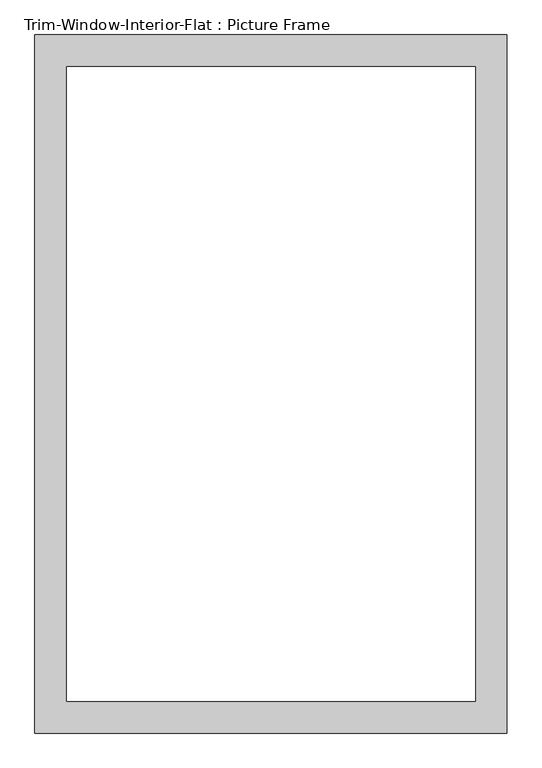
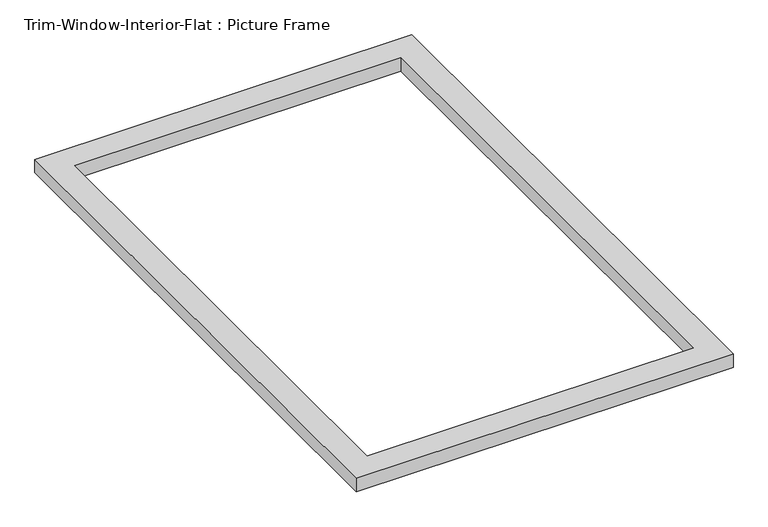
"""IFC4 building model written with IfcOpenShell, lengths in millimetres: proxy geometry, Trim-Window-Interior-Flat : Picture Frame."""

from ifc_helpers import new_model, si_unit, origin, origin_with_axes, place, context, project, spatial, polyline, outline, extrude, source, transform, mapped, element, save


def trim_window_interior_flat_picture_frame_840a62db(model_context):
    return source(origin(), model_context, "Body", "SweptSolid", [
        extrude(outline(polyline([(425.45, 44.45), (425.45, -1212.85), (-425.45, -1212.85), (-425.45, 44.45), (425.45, 44.45)]), holes=[polyline([(368.3, -12.7), (-368.3, -12.7), (-368.3, -1155.7), (368.3, -1155.7), (368.3, -12.7)])]), origin_with_axes(), (0.0, 0.0, 1.0), 31.75),
    ])


if __name__ == "__main__":
    model = new_model("IFC4")
    model_context = context("Model", 3, world=origin())
    ifc_project = project(units=[si_unit("LENGTHUNIT", "METRE", prefix="MILLI")], contexts=[model_context])
    site = spatial("IfcSite", under=ifc_project)
    building = spatial("IfcBuilding", under=site)
    placement = place(None, origin())
    trim_window_interior_flat_picture_frame_shape = trim_window_interior_flat_picture_frame_840a62db(model_context)
    element("IfcBuildingElementProxy", 1, Name="Trim-Window-Interior-Flat : Picture Frame", ObjectType="Trim-Window-Interior-Flat : Picture Frame", at=placement, inside=building, context=model_context, shape_type="MappedRepresentation", body=[
        mapped(trim_window_interior_flat_picture_frame_shape, transform((0.0, 0.0, 0.0), x_axis=(1.0, 0.0, 0.0), y_axis=(0.0, 1.0, 0.0), z_axis=(0.0, 0.0, 1.0))),
    ])
    save(model, "model.ifc")

# Revit data of these elements
# Type "Trim-Window-Interior-Flat : Picture Frame"
#   Trim Thickness_Picture Frame = 0' - 1 1/4"
#   Trim Width = 0' - 2 1/4"
#   Trim Thickness_with Sill = 0' - 0 3/4"
#   Sill Thickness = 0' - 1 1/4"
#   Opening Width [instance default] = 2' - 0"
#   Opening Height [instance default] = 3' - 0"
#   Default Elevation = 4' - 0"
#   Sill = no
#   Picture Frame = yes
#   Trim Material [instance default] = none
# Element 1 (IfcBuildingElementProxy, "Trim-Window-Interior-Flat : Picture Frame")
#   Opening Width = 2' - 6"
#   Opening Height = 3' - 10"
#   Trim Material = Wood - Stained
#   Materials on its faces: "Wood - Stained"
# Materials
#   "Wood - Stained": class "Wood", colour RGB 224 178 126, transparency 0, Cost = 0
